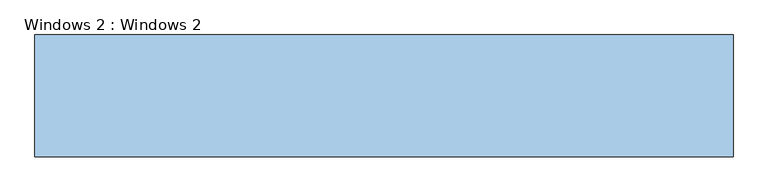
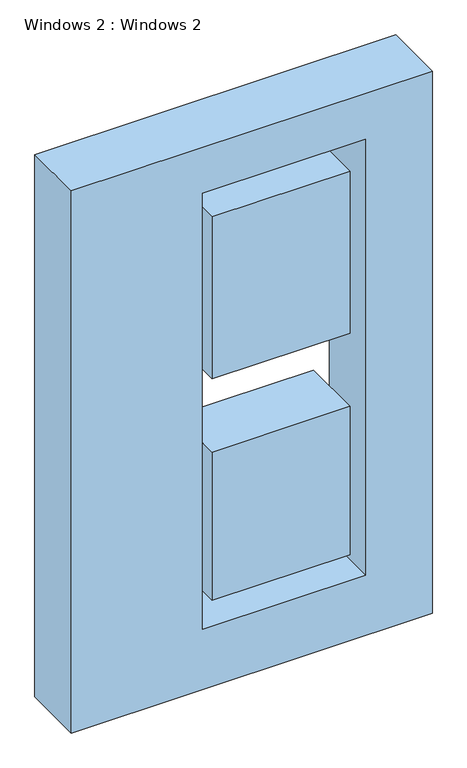
"""IFC4 building model written with IfcOpenShell, lengths in millimetres: window geometry, Windows 2 : Windows 2."""

from ifc_helpers import new_model, si_unit, frame, origin, place, context, project, spatial, polyline, outline, extrude, source, transform, mapped, element, save


def windows_2_windows_2_da26fb5b(model_context):
    return source(origin(), model_context, "Body", "SweptSolid", [
        extrude(outline(polyline([(11663.1283634, -1302.079547), (11663.1283634, -8902.079547), (-400.0, -8902.079547), (-400.0, -1302.079547), (11663.1283634, -1302.079547)]), holes=[polyline([(10641.3308609, -2703.3852997), (941.3308609, -2703.3852997), (941.3308609, -6132.4876142), (10641.3308609, -6132.4876142), (10641.3308609, -2703.3852997)])]), frame((0.0, -10393.2199515, 0.0), z_axis=(0.0, 1.0, 0.0), x_axis=(0.0, 0.0, 1.0)), (0.0, 0.0, 1.0), 1326.8191547),
        extrude(outline(polyline([(-5938.19828, -9066.4007969), (-3038.19828, -9066.4007969), (-3038.19828, -10393.2199515), (-5938.19828, -10393.2199515), (-5938.19828, -9066.4007969)])), frame((0.0, 0.0, 6444.8843334), z_axis=(0.0, 0.0, 1.0), x_axis=(1.0, 0.0, 0.0)), (0.0, 0.0, 1.0), 3600.0),
        extrude(outline(polyline([(-5938.19828, -9066.4007969), (-3038.19828, -9066.4007969), (-3038.19828, -10393.2199515), (-5938.19828, -10393.2199515), (-5938.19828, -9066.4007969)])), frame((0.0, 0.0, 1518.2079254), z_axis=(0.0, 0.0, 1.0), x_axis=(1.0, 0.0, 0.0)), (0.0, 0.0, 1.0), 3292.9183867),
    ])


if __name__ == "__main__":
    model = new_model("IFC4")
    model_context = context("Model", 3, world=origin())
    ifc_project = project(units=[si_unit("LENGTHUNIT", "METRE", prefix="MILLI")], contexts=[model_context])
    site = spatial("IfcSite", under=ifc_project)
    building = spatial("IfcBuilding", under=site)
    placement = place(None, origin())
    windows_2_windows_2_shape = windows_2_windows_2_da26fb5b(model_context)
    element("IfcWindow", 1, ObjectType="Windows 2 : Windows 2", at=placement, inside=building, context=model_context, shape_type="MappedRepresentation", body=[
        mapped(windows_2_windows_2_shape, transform((0.0, 0.0, 0.0), x_axis=(1.0, 0.0, 0.0), y_axis=(0.0, 1.0, 0.0), z_axis=(0.0, 0.0, 1.0))),
    ])
    save(model, "model.ifc")

# Revit data of these elements
# Type "Windows 2 : Windows 2"
#   Type Mark = "23"
